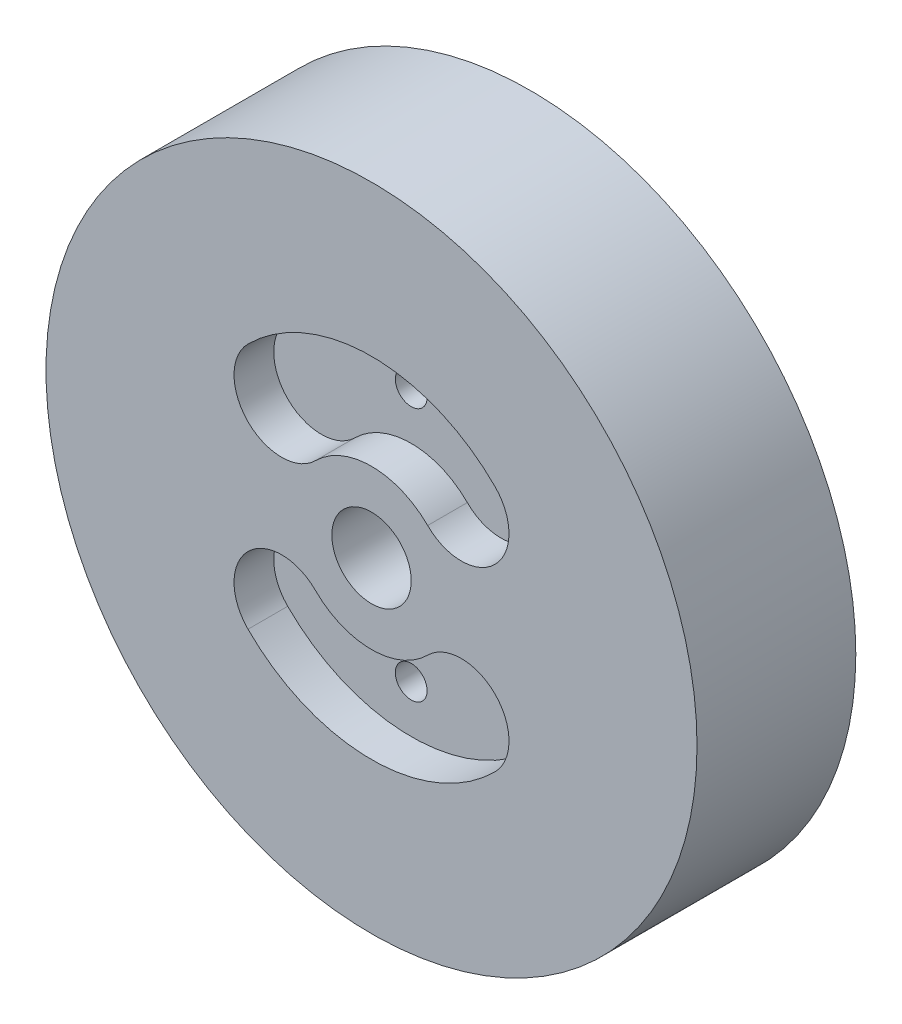
ISO-10303-21;
HEADER;
FILE_DESCRIPTION(('STEP AP214'),'2;1');
FILE_NAME('part.step','',(''),(''),'','','');
FILE_SCHEMA(('AUTOMOTIVE_DESIGN { 1 0 10303 214 1 1 1 1 }'));
ENDSEC;
DATA;
#1=APPLICATION_CONTEXT('core data for automotive mechanical design processes');
#2=APPLICATION_PROTOCOL_DEFINITION('international standard','automotive_design',2000,#1);
#3=PRODUCT_CONTEXT('',#1,'mechanical');
#4=PRODUCT('Part','Part','',(#3));
#5=PRODUCT_RELATED_PRODUCT_CATEGORY('part','',(#4));
#6=PRODUCT_DEFINITION_FORMATION('','',#4);
#7=PRODUCT_DEFINITION_CONTEXT('part definition',#1,'design');
#8=PRODUCT_DEFINITION('design','',#6,#7);
#9=PRODUCT_DEFINITION_SHAPE('','',#8);
#10=(LENGTH_UNIT() NAMED_UNIT(*) SI_UNIT(.MILLI.,.METRE.));
#11=(NAMED_UNIT(*) PLANE_ANGLE_UNIT() SI_UNIT($,.RADIAN.));
#12=(NAMED_UNIT(*) SI_UNIT($,.STERADIAN.) SOLID_ANGLE_UNIT());
#13=UNCERTAINTY_MEASURE_WITH_UNIT(LENGTH_MEASURE(1.E-05),#10,'distance_accuracy_value','');
#14=(GEOMETRIC_REPRESENTATION_CONTEXT(3) GLOBAL_UNCERTAINTY_ASSIGNED_CONTEXT((#13)) GLOBAL_UNIT_ASSIGNED_CONTEXT((#10,
#11,#12)) REPRESENTATION_CONTEXT('',''));
#15=CARTESIAN_POINT('',(0.,0.,0.));
#16=DIRECTION('',(0.,0.,1.));
#17=DIRECTION('',(1.,0.,0.));
#18=AXIS2_PLACEMENT_3D('',#15,#16,#17);
#19=CARTESIAN_POINT('',(0.,0.,10.));
#20=DIRECTION('',(0.,0.,-1.));
#21=DIRECTION('',(-1.,0.,0.));
#22=AXIS2_PLACEMENT_3D('',#19,#20,#21);
#23=CYLINDRICAL_SURFACE('',#22,20.5);
#24=CARTESIAN_POINT('',(0.,0.,10.));
#25=DIRECTION('',(0.,0.,1.));
#26=DIRECTION('',(1.,0.,0.));
#27=AXIS2_PLACEMENT_3D('',#24,#25,#26);
#28=CIRCLE('',#27,20.5);
#29=CARTESIAN_POINT('',(20.5,0.,10.));
#30=VERTEX_POINT('',#29);
#31=EDGE_CURVE('E11',#30,#30,#28,.T.);
#32=ORIENTED_EDGE('',*,*,#31,.F.);
#33=EDGE_LOOP('',(#32));
#34=FACE_BOUND('',#33,.T.);
#35=CARTESIAN_POINT('',(0.,0.,0.));
#36=DIRECTION('',(0.,0.,1.));
#37=DIRECTION('',(1.,0.,0.));
#38=AXIS2_PLACEMENT_3D('',#35,#36,#37);
#39=CIRCLE('',#38,20.5);
#40=CARTESIAN_POINT('',(20.5,0.,0.));
#41=VERTEX_POINT('',#40);
#42=EDGE_CURVE('E52',#41,#41,#39,.T.);
#43=ORIENTED_EDGE('',*,*,#42,.T.);
#44=EDGE_LOOP('',(#43));
#45=FACE_BOUND('',#44,.T.);
#46=ADVANCED_FACE('F44',(#34,#45),#23,.T.);
#47=CARTESIAN_POINT('',(0.,0.,10.));
#48=DIRECTION('',(0.,0.,1.));
#49=DIRECTION('',(1.,0.,0.));
#50=AXIS2_PLACEMENT_3D('',#47,#48,#49);
#51=PLANE('',#50);
#52=CARTESIAN_POINT('',(0.,0.,10.));
#53=DIRECTION('',(0.,0.,1.));
#54=DIRECTION('',(1.,0.,0.));
#55=AXIS2_PLACEMENT_3D('',#52,#53,#54);
#56=CIRCLE('',#55,2.5);
#57=CARTESIAN_POINT('',(2.5,0.,10.));
#58=VERTEX_POINT('',#57);
#59=EDGE_CURVE('E190',#58,#58,#56,.T.);
#60=ORIENTED_EDGE('',*,*,#59,.F.);
#61=EDGE_LOOP('',(#60));
#62=FACE_BOUND('',#61,.T.);
#63=CARTESIAN_POINT('',(5.65685424949237,-5.65685424949239,10.));
#64=DIRECTION('',(0.,0.,1.));
#65=DIRECTION('',(-1.,0.,0.));
#66=AXIS2_PLACEMENT_3D('',#63,#64,#65);
#67=CIRCLE('',#66,3.);
#68=CARTESIAN_POINT('',(7.77817459305201,-7.77817459305204,10.));
#69=VERTEX_POINT('',#68);
#70=CARTESIAN_POINT('',(3.53553390593273,-3.53553390593274,10.));
#71=VERTEX_POINT('',#70);
#72=EDGE_CURVE('E61',#69,#71,#67,.T.);
#73=ORIENTED_EDGE('',*,*,#72,.F.);
#74=CARTESIAN_POINT('',(0.,0.,10.));
#75=DIRECTION('',(0.,0.,1.));
#76=DIRECTION('',(-1.,0.,0.));
#77=AXIS2_PLACEMENT_3D('',#74,#75,#76);
#78=CIRCLE('',#77,11.);
#79=CARTESIAN_POINT('',(-7.77817459305201,-7.77817459305204,10.));
#80=VERTEX_POINT('',#79);
#81=EDGE_CURVE('E131',#80,#69,#78,.T.);
#82=ORIENTED_EDGE('',*,*,#81,.F.);
#83=CARTESIAN_POINT('',(-5.65685424949237,-5.65685424949239,10.));
#84=DIRECTION('',(0.,0.,1.));
#85=DIRECTION('',(1.,0.,0.));
#86=AXIS2_PLACEMENT_3D('',#83,#84,#85);
#87=CIRCLE('',#86,3.);
#88=CARTESIAN_POINT('',(-3.53553390593273,-3.53553390593275,10.));
#89=VERTEX_POINT('',#88);
#90=EDGE_CURVE('E133',#89,#80,#87,.T.);
#91=ORIENTED_EDGE('',*,*,#90,.F.);
#92=CARTESIAN_POINT('',(0.,0.,10.));
#93=DIRECTION('',(0.,0.,-1.));
#94=DIRECTION('',(-1.,0.,0.));
#95=AXIS2_PLACEMENT_3D('',#92,#93,#94);
#96=CIRCLE('',#95,5.);
#97=EDGE_CURVE('E141',#71,#89,#96,.T.);
#98=ORIENTED_EDGE('',*,*,#97,.F.);
#99=EDGE_LOOP('',(#73,#82,#91,#98));
#100=FACE_BOUND('',#99,.T.);
#101=CARTESIAN_POINT('',(5.65685424949237,5.65685424949239,10.));
#102=DIRECTION('',(0.,0.,1.));
#103=DIRECTION('',(1.,0.,0.));
#104=AXIS2_PLACEMENT_3D('',#101,#102,#103);
#105=CIRCLE('',#104,3.);
#106=CARTESIAN_POINT('',(3.53553390593273,3.53553390593274,10.));
#107=VERTEX_POINT('',#106);
#108=CARTESIAN_POINT('',(7.778174593052,7.77817459305204,10.));
#109=VERTEX_POINT('',#108);
#110=EDGE_CURVE('E66',#107,#109,#105,.T.);
#111=ORIENTED_EDGE('',*,*,#110,.F.);
#112=CARTESIAN_POINT('',(0.,0.,10.));
#113=DIRECTION('',(0.,0.,-1.));
#114=DIRECTION('',(1.,0.,0.));
#115=AXIS2_PLACEMENT_3D('',#112,#113,#114);
#116=CIRCLE('',#115,5.);
#117=CARTESIAN_POINT('',(-3.53553390593273,3.53553390593275,10.));
#118=VERTEX_POINT('',#117);
#119=EDGE_CURVE('E160',#118,#107,#116,.T.);
#120=ORIENTED_EDGE('',*,*,#119,.F.);
#121=CARTESIAN_POINT('',(-5.65685424949237,5.65685424949239,10.));
#122=DIRECTION('',(0.,0.,1.));
#123=DIRECTION('',(-1.,0.,0.));
#124=AXIS2_PLACEMENT_3D('',#121,#122,#123);
#125=CIRCLE('',#124,3.);
#126=CARTESIAN_POINT('',(-7.778174593052,7.77817459305204,10.));
#127=VERTEX_POINT('',#126);
#128=EDGE_CURVE('E171',#127,#118,#125,.T.);
#129=ORIENTED_EDGE('',*,*,#128,.F.);
#130=CARTESIAN_POINT('',(0.,0.,10.));
#131=DIRECTION('',(0.,0.,1.));
#132=DIRECTION('',(1.,0.,0.));
#133=AXIS2_PLACEMENT_3D('',#130,#131,#132);
#134=CIRCLE('',#133,11.);
#135=EDGE_CURVE('E169',#109,#127,#134,.T.);
#136=ORIENTED_EDGE('',*,*,#135,.F.);
#137=EDGE_LOOP('',(#111,#120,#129,#136));
#138=FACE_BOUND('',#137,.T.);
#139=ORIENTED_EDGE('',*,*,#31,.T.);
#140=EDGE_LOOP('',(#139));
#141=FACE_BOUND('',#140,.T.);
#142=ADVANCED_FACE('F223',(#62,#100,#138,#141),#51,.T.);
#143=CARTESIAN_POINT('',(0.,0.,0.));
#144=DIRECTION('',(0.,0.,1.));
#145=DIRECTION('',(1.,0.,0.));
#146=AXIS2_PLACEMENT_3D('',#143,#144,#145);
#147=PLANE('',#146);
#148=CARTESIAN_POINT('',(-12.5,0.,0.));
#149=DIRECTION('',(0.,0.,-1.));
#150=DIRECTION('',(-1.,0.,0.));
#151=AXIS2_PLACEMENT_3D('',#148,#149,#150);
#152=CIRCLE('',#151,2.5);
#153=CARTESIAN_POINT('',(-15.,0.,0.));
#154=VERTEX_POINT('',#153);
#155=EDGE_CURVE('E206',#154,#154,#152,.T.);
#156=ORIENTED_EDGE('',*,*,#155,.F.);
#157=EDGE_LOOP('',(#156));
#158=FACE_BOUND('',#157,.T.);
#159=CARTESIAN_POINT('',(12.5,0.,0.));
#160=DIRECTION('',(0.,0.,-1.));
#161=DIRECTION('',(-1.,0.,0.));
#162=AXIS2_PLACEMENT_3D('',#159,#160,#161);
#163=CIRCLE('',#162,2.5);
#164=CARTESIAN_POINT('',(10.,0.,0.));
#165=VERTEX_POINT('',#164);
#166=EDGE_CURVE('E199',#165,#165,#163,.T.);
#167=ORIENTED_EDGE('',*,*,#166,.F.);
#168=EDGE_LOOP('',(#167));
#169=FACE_BOUND('',#168,.T.);
#170=CARTESIAN_POINT('',(0.,-8.,0.));
#171=DIRECTION('',(0.,0.,1.));
#172=DIRECTION('',(1.,0.,0.));
#173=AXIS2_PLACEMENT_3D('',#170,#171,#172);
#174=CIRCLE('',#173,1.);
#175=CARTESIAN_POINT('',(1.,-8.,0.));
#176=VERTEX_POINT('',#175);
#177=EDGE_CURVE('E186',#176,#176,#174,.T.);
#178=ORIENTED_EDGE('',*,*,#177,.T.);
#179=EDGE_LOOP('',(#178));
#180=FACE_BOUND('',#179,.T.);
#181=CARTESIAN_POINT('',(0.,8.,0.));
#182=DIRECTION('',(0.,0.,1.));
#183=DIRECTION('',(1.,0.,0.));
#184=AXIS2_PLACEMENT_3D('',#181,#182,#183);
#185=CIRCLE('',#184,1.);
#186=CARTESIAN_POINT('',(1.,8.,0.));
#187=VERTEX_POINT('',#186);
#188=EDGE_CURVE('E139',#187,#187,#185,.T.);
#189=ORIENTED_EDGE('',*,*,#188,.T.);
#190=EDGE_LOOP('',(#189));
#191=FACE_BOUND('',#190,.T.);
#192=CARTESIAN_POINT('',(0.,0.,0.));
#193=DIRECTION('',(0.,0.,1.));
#194=DIRECTION('',(1.,0.,0.));
#195=AXIS2_PLACEMENT_3D('',#192,#193,#194);
#196=CIRCLE('',#195,2.5);
#197=CARTESIAN_POINT('',(2.5,0.,0.));
#198=VERTEX_POINT('',#197);
#199=EDGE_CURVE('E48',#198,#198,#196,.T.);
#200=ORIENTED_EDGE('',*,*,#199,.T.);
#201=EDGE_LOOP('',(#200));
#202=FACE_BOUND('',#201,.T.);
#203=ORIENTED_EDGE('',*,*,#42,.F.);
#204=EDGE_LOOP('',(#203));
#205=FACE_BOUND('',#204,.T.);
#206=ADVANCED_FACE('F222',(#158,#169,#180,#191,#202,#205),#147,.F.);
#207=CARTESIAN_POINT('',(5.65685424949237,5.65685424949239,7.5));
#208=DIRECTION('',(0.,0.,1.));
#209=DIRECTION('',(1.,0.,0.));
#210=AXIS2_PLACEMENT_3D('',#207,#208,#209);
#211=CYLINDRICAL_SURFACE('',#210,3.);
#212=ORIENTED_EDGE('',*,*,#110,.T.);
#213=DIRECTION('',(0.,0.,1.));
#214=VECTOR('',#213,1.);
#215=CARTESIAN_POINT('',(7.778174593052,7.77817459305204,7.5));
#216=LINE('',#215,#214);
#217=CARTESIAN_POINT('',(7.778174593052,7.77817459305204,7.5));
#218=VERTEX_POINT('',#217);
#219=EDGE_CURVE('E167',#218,#109,#216,.T.);
#220=ORIENTED_EDGE('',*,*,#219,.F.);
#221=CARTESIAN_POINT('',(5.65685424949237,5.65685424949239,7.5));
#222=DIRECTION('',(0.,0.,1.));
#223=DIRECTION('',(1.,0.,0.));
#224=AXIS2_PLACEMENT_3D('',#221,#222,#223);
#225=CIRCLE('',#224,3.);
#226=CARTESIAN_POINT('',(3.53553390593273,3.53553390593274,7.5));
#227=VERTEX_POINT('',#226);
#228=EDGE_CURVE('E153',#227,#218,#225,.T.);
#229=ORIENTED_EDGE('',*,*,#228,.F.);
#230=DIRECTION('',(0.,0.,1.));
#231=VECTOR('',#230,1.);
#232=CARTESIAN_POINT('',(3.53553390593273,3.53553390593274,7.5));
#233=LINE('',#232,#231);
#234=EDGE_CURVE('E145',#227,#107,#233,.T.);
#235=ORIENTED_EDGE('',*,*,#234,.T.);
#236=EDGE_LOOP('',(#212,#220,#229,#235));
#237=FACE_BOUND('',#236,.T.);
#238=ADVANCED_FACE('F221',(#237),#211,.F.);
#239=CARTESIAN_POINT('',(0.,0.,7.5));
#240=DIRECTION('',(0.,0.,1.));
#241=DIRECTION('',(1.,0.,0.));
#242=AXIS2_PLACEMENT_3D('',#239,#240,#241);
#243=CYLINDRICAL_SURFACE('',#242,5.);
#244=ORIENTED_EDGE('',*,*,#119,.T.);
#245=ORIENTED_EDGE('',*,*,#234,.F.);
#246=CARTESIAN_POINT('',(0.,0.,7.5));
#247=DIRECTION('',(0.,0.,-1.));
#248=DIRECTION('',(1.,0.,0.));
#249=AXIS2_PLACEMENT_3D('',#246,#247,#248);
#250=CIRCLE('',#249,5.);
#251=CARTESIAN_POINT('',(-3.53553390593273,3.53553390593275,7.5));
#252=VERTEX_POINT('',#251);
#253=EDGE_CURVE('E162',#252,#227,#250,.T.);
#254=ORIENTED_EDGE('',*,*,#253,.F.);
#255=DIRECTION('',(0.,0.,1.));
#256=VECTOR('',#255,1.);
#257=CARTESIAN_POINT('',(-3.53553390593273,3.53553390593275,7.5));
#258=LINE('',#257,#256);
#259=EDGE_CURVE('E179',#252,#118,#258,.T.);
#260=ORIENTED_EDGE('',*,*,#259,.T.);
#261=EDGE_LOOP('',(#244,#245,#254,#260));
#262=FACE_BOUND('',#261,.T.);
#263=ADVANCED_FACE('F255',(#262),#243,.T.);
#264=CARTESIAN_POINT('',(-5.65685424949237,5.65685424949239,7.5));
#265=DIRECTION('',(0.,0.,1.));
#266=DIRECTION('',(1.,0.,0.));
#267=AXIS2_PLACEMENT_3D('',#264,#265,#266);
#268=CYLINDRICAL_SURFACE('',#267,3.);
#269=ORIENTED_EDGE('',*,*,#128,.T.);
#270=ORIENTED_EDGE('',*,*,#259,.F.);
#271=CARTESIAN_POINT('',(-5.65685424949237,5.65685424949239,7.5));
#272=DIRECTION('',(0.,0.,1.));
#273=DIRECTION('',(-1.,0.,0.));
#274=AXIS2_PLACEMENT_3D('',#271,#272,#273);
#275=CIRCLE('',#274,3.);
#276=CARTESIAN_POINT('',(-7.778174593052,7.77817459305204,7.5));
#277=VERTEX_POINT('',#276);
#278=EDGE_CURVE('E159',#277,#252,#275,.T.);
#279=ORIENTED_EDGE('',*,*,#278,.F.);
#280=DIRECTION('',(0.,0.,1.));
#281=VECTOR('',#280,1.);
#282=CARTESIAN_POINT('',(-7.778174593052,7.77817459305204,7.5));
#283=LINE('',#282,#281);
#284=EDGE_CURVE('E176',#277,#127,#283,.T.);
#285=ORIENTED_EDGE('',*,*,#284,.T.);
#286=EDGE_LOOP('',(#269,#270,#279,#285));
#287=FACE_BOUND('',#286,.T.);
#288=ADVANCED_FACE('F259',(#287),#268,.F.);
#289=CARTESIAN_POINT('',(0.,0.,7.5));
#290=DIRECTION('',(0.,0.,1.));
#291=DIRECTION('',(1.,0.,0.));
#292=AXIS2_PLACEMENT_3D('',#289,#290,#291);
#293=CYLINDRICAL_SURFACE('',#292,11.);
#294=ORIENTED_EDGE('',*,*,#135,.T.);
#295=ORIENTED_EDGE('',*,*,#284,.F.);
#296=CARTESIAN_POINT('',(0.,0.,7.5));
#297=DIRECTION('',(0.,0.,1.));
#298=DIRECTION('',(1.,0.,0.));
#299=AXIS2_PLACEMENT_3D('',#296,#297,#298);
#300=CIRCLE('',#299,11.);
#301=EDGE_CURVE('E156',#218,#277,#300,.T.);
#302=ORIENTED_EDGE('',*,*,#301,.F.);
#303=ORIENTED_EDGE('',*,*,#219,.T.);
#304=EDGE_LOOP('',(#294,#295,#302,#303));
#305=FACE_BOUND('',#304,.T.);
#306=ADVANCED_FACE('F254',(#305),#293,.F.);
#307=CARTESIAN_POINT('',(2.82842712474618,2.8284271247462,7.5));
#308=DIRECTION('',(0.,0.,1.));
#309=DIRECTION('',(1.,0.,0.));
#310=AXIS2_PLACEMENT_3D('',#307,#308,#309);
#311=PLANE('',#310);
#312=CARTESIAN_POINT('',(0.,8.,7.5));
#313=DIRECTION('',(0.,0.,1.));
#314=DIRECTION('',(1.,0.,0.));
#315=AXIS2_PLACEMENT_3D('',#312,#313,#314);
#316=CIRCLE('',#315,1.);
#317=CARTESIAN_POINT('',(1.,8.,7.5));
#318=VERTEX_POINT('',#317);
#319=EDGE_CURVE('E187',#318,#318,#316,.T.);
#320=ORIENTED_EDGE('',*,*,#319,.F.);
#321=EDGE_LOOP('',(#320));
#322=FACE_BOUND('',#321,.T.);
#323=ORIENTED_EDGE('',*,*,#228,.T.);
#324=ORIENTED_EDGE('',*,*,#301,.T.);
#325=ORIENTED_EDGE('',*,*,#278,.T.);
#326=ORIENTED_EDGE('',*,*,#253,.T.);
#327=EDGE_LOOP('',(#323,#324,#325,#326));
#328=FACE_BOUND('',#327,.T.);
#329=ADVANCED_FACE('F256',(#322,#328),#311,.T.);
#330=CARTESIAN_POINT('',(5.65685424949237,-5.65685424949239,7.5));
#331=DIRECTION('',(0.,0.,1.));
#332=DIRECTION('',(1.,0.,0.));
#333=AXIS2_PLACEMENT_3D('',#330,#331,#332);
#334=CYLINDRICAL_SURFACE('',#333,3.);
#335=ORIENTED_EDGE('',*,*,#72,.T.);
#336=DIRECTION('',(0.,0.,1.));
#337=VECTOR('',#336,1.);
#338=CARTESIAN_POINT('',(3.53553390593273,-3.53553390593274,7.5));
#339=LINE('',#338,#337);
#340=CARTESIAN_POINT('',(3.53553390593273,-3.53553390593274,7.5));
#341=VERTEX_POINT('',#340);
#342=EDGE_CURVE('E108',#341,#71,#339,.T.);
#343=ORIENTED_EDGE('',*,*,#342,.F.);
#344=CARTESIAN_POINT('',(5.65685424949237,-5.65685424949239,7.5));
#345=DIRECTION('',(0.,0.,1.));
#346=DIRECTION('',(-1.,0.,0.));
#347=AXIS2_PLACEMENT_3D('',#344,#345,#346);
#348=CIRCLE('',#347,3.);
#349=CARTESIAN_POINT('',(7.77817459305201,-7.77817459305204,7.5));
#350=VERTEX_POINT('',#349);
#351=EDGE_CURVE('E114',#350,#341,#348,.T.);
#352=ORIENTED_EDGE('',*,*,#351,.F.);
#353=DIRECTION('',(0.,0.,1.));
#354=VECTOR('',#353,1.);
#355=CARTESIAN_POINT('',(7.77817459305201,-7.77817459305204,7.5));
#356=LINE('',#355,#354);
#357=EDGE_CURVE('E146',#350,#69,#356,.T.);
#358=ORIENTED_EDGE('',*,*,#357,.T.);
#359=EDGE_LOOP('',(#335,#343,#352,#358));
#360=FACE_BOUND('',#359,.T.);
#361=ADVANCED_FACE('F112',(#360),#334,.F.);
#362=CARTESIAN_POINT('',(0.,0.,7.5));
#363=DIRECTION('',(0.,0.,1.));
#364=DIRECTION('',(1.,0.,0.));
#365=AXIS2_PLACEMENT_3D('',#362,#363,#364);
#366=CYLINDRICAL_SURFACE('',#365,11.);
#367=ORIENTED_EDGE('',*,*,#81,.T.);
#368=ORIENTED_EDGE('',*,*,#357,.F.);
#369=CARTESIAN_POINT('',(0.,0.,7.5));
#370=DIRECTION('',(0.,0.,1.));
#371=DIRECTION('',(-1.,0.,0.));
#372=AXIS2_PLACEMENT_3D('',#369,#370,#371);
#373=CIRCLE('',#372,11.);
#374=CARTESIAN_POINT('',(-7.77817459305201,-7.77817459305204,7.5));
#375=VERTEX_POINT('',#374);
#376=EDGE_CURVE('E118',#375,#350,#373,.T.);
#377=ORIENTED_EDGE('',*,*,#376,.F.);
#378=DIRECTION('',(0.,0.,1.));
#379=VECTOR('',#378,1.);
#380=CARTESIAN_POINT('',(-7.77817459305201,-7.77817459305204,7.5));
#381=LINE('',#380,#379);
#382=EDGE_CURVE('E147',#375,#80,#381,.T.);
#383=ORIENTED_EDGE('',*,*,#382,.T.);
#384=EDGE_LOOP('',(#367,#368,#377,#383));
#385=FACE_BOUND('',#384,.T.);
#386=ADVANCED_FACE('F275',(#385),#366,.F.);
#387=CARTESIAN_POINT('',(-5.65685424949237,-5.65685424949239,7.5));
#388=DIRECTION('',(0.,0.,1.));
#389=DIRECTION('',(1.,0.,0.));
#390=AXIS2_PLACEMENT_3D('',#387,#388,#389);
#391=CYLINDRICAL_SURFACE('',#390,3.);
#392=ORIENTED_EDGE('',*,*,#90,.T.);
#393=ORIENTED_EDGE('',*,*,#382,.F.);
#394=CARTESIAN_POINT('',(-5.65685424949237,-5.65685424949239,7.5));
#395=DIRECTION('',(0.,0.,1.));
#396=DIRECTION('',(1.,0.,0.));
#397=AXIS2_PLACEMENT_3D('',#394,#395,#396);
#398=CIRCLE('',#397,3.);
#399=CARTESIAN_POINT('',(-3.53553390593273,-3.53553390593275,7.5));
#400=VERTEX_POINT('',#399);
#401=EDGE_CURVE('E130',#400,#375,#398,.T.);
#402=ORIENTED_EDGE('',*,*,#401,.F.);
#403=DIRECTION('',(0.,0.,1.));
#404=VECTOR('',#403,1.);
#405=CARTESIAN_POINT('',(-3.53553390593273,-3.53553390593275,7.5));
#406=LINE('',#405,#404);
#407=EDGE_CURVE('E117',#400,#89,#406,.T.);
#408=ORIENTED_EDGE('',*,*,#407,.T.);
#409=EDGE_LOOP('',(#392,#393,#402,#408));
#410=FACE_BOUND('',#409,.T.);
#411=ADVANCED_FACE('F273',(#410),#391,.F.);
#412=CARTESIAN_POINT('',(0.,0.,7.5));
#413=DIRECTION('',(0.,0.,1.));
#414=DIRECTION('',(1.,0.,0.));
#415=AXIS2_PLACEMENT_3D('',#412,#413,#414);
#416=CYLINDRICAL_SURFACE('',#415,5.);
#417=ORIENTED_EDGE('',*,*,#97,.T.);
#418=ORIENTED_EDGE('',*,*,#407,.F.);
#419=CARTESIAN_POINT('',(0.,0.,7.5));
#420=DIRECTION('',(0.,0.,-1.));
#421=DIRECTION('',(-1.,0.,0.));
#422=AXIS2_PLACEMENT_3D('',#419,#420,#421);
#423=CIRCLE('',#422,5.);
#424=EDGE_CURVE('E124',#341,#400,#423,.T.);
#425=ORIENTED_EDGE('',*,*,#424,.F.);
#426=ORIENTED_EDGE('',*,*,#342,.T.);
#427=EDGE_LOOP('',(#417,#418,#425,#426));
#428=FACE_BOUND('',#427,.T.);
#429=ADVANCED_FACE('F125',(#428),#416,.T.);
#430=CARTESIAN_POINT('',(2.82842712474618,-2.8284271247462,7.5));
#431=DIRECTION('',(0.,0.,-1.));
#432=DIRECTION('',(-1.,0.,0.));
#433=AXIS2_PLACEMENT_3D('',#430,#431,#432);
#434=PLANE('',#433);
#435=CARTESIAN_POINT('',(0.,-8.,7.5));
#436=DIRECTION('',(0.,0.,-1.));
#437=DIRECTION('',(-1.,0.,0.));
#438=AXIS2_PLACEMENT_3D('',#435,#436,#437);
#439=CIRCLE('',#438,1.);
#440=CARTESIAN_POINT('',(-1.,-8.,7.5));
#441=VERTEX_POINT('',#440);
#442=EDGE_CURVE('E184',#441,#441,#439,.T.);
#443=ORIENTED_EDGE('',*,*,#442,.T.);
#444=EDGE_LOOP('',(#443));
#445=FACE_BOUND('',#444,.T.);
#446=ORIENTED_EDGE('',*,*,#351,.T.);
#447=ORIENTED_EDGE('',*,*,#424,.T.);
#448=ORIENTED_EDGE('',*,*,#401,.T.);
#449=ORIENTED_EDGE('',*,*,#376,.T.);
#450=EDGE_LOOP('',(#446,#447,#448,#449));
#451=FACE_BOUND('',#450,.T.);
#452=ADVANCED_FACE('F129',(#445,#451),#434,.F.);
#453=CARTESIAN_POINT('',(0.,-8.,-22.5));
#454=DIRECTION('',(0.,0.,1.));
#455=DIRECTION('',(1.,0.,0.));
#456=AXIS2_PLACEMENT_3D('',#453,#454,#455);
#457=CYLINDRICAL_SURFACE('',#456,1.);
#458=ORIENTED_EDGE('',*,*,#442,.F.);
#459=EDGE_LOOP('',(#458));
#460=FACE_BOUND('',#459,.T.);
#461=ORIENTED_EDGE('',*,*,#177,.F.);
#462=EDGE_LOOP('',(#461));
#463=FACE_BOUND('',#462,.T.);
#464=ADVANCED_FACE('F282',(#460,#463),#457,.F.);
#465=CARTESIAN_POINT('',(0.,8.,-22.5));
#466=DIRECTION('',(0.,0.,1.));
#467=DIRECTION('',(1.,0.,0.));
#468=AXIS2_PLACEMENT_3D('',#465,#466,#467);
#469=CYLINDRICAL_SURFACE('',#468,1.);
#470=ORIENTED_EDGE('',*,*,#319,.T.);
#471=EDGE_LOOP('',(#470));
#472=FACE_BOUND('',#471,.T.);
#473=ORIENTED_EDGE('',*,*,#188,.F.);
#474=EDGE_LOOP('',(#473));
#475=FACE_BOUND('',#474,.T.);
#476=ADVANCED_FACE('F286',(#472,#475),#469,.F.);
#477=CARTESIAN_POINT('',(0.,0.,-22.5));
#478=DIRECTION('',(0.,0.,1.));
#479=DIRECTION('',(1.,0.,0.));
#480=AXIS2_PLACEMENT_3D('',#477,#478,#479);
#481=CYLINDRICAL_SURFACE('',#480,2.5);
#482=ORIENTED_EDGE('',*,*,#59,.T.);
#483=EDGE_LOOP('',(#482));
#484=FACE_BOUND('',#483,.T.);
#485=ORIENTED_EDGE('',*,*,#199,.F.);
#486=EDGE_LOOP('',(#485));
#487=FACE_BOUND('',#486,.T.);
#488=ADVANCED_FACE('F284',(#484,#487),#481,.F.);
#489=CARTESIAN_POINT('',(12.5,0.,5.));
#490=DIRECTION('',(0.,0.,-1.));
#491=DIRECTION('',(-1.,0.,0.));
#492=AXIS2_PLACEMENT_3D('',#489,#490,#491);
#493=CYLINDRICAL_SURFACE('',#492,2.5);
#494=CARTESIAN_POINT('',(12.5,0.,5.));
#495=DIRECTION('',(0.,0.,-1.));
#496=DIRECTION('',(-1.,0.,0.));
#497=AXIS2_PLACEMENT_3D('',#494,#495,#496);
#498=CIRCLE('',#497,2.5);
#499=CARTESIAN_POINT('',(10.,0.,5.));
#500=VERTEX_POINT('',#499);
#501=EDGE_CURVE('E201',#500,#500,#498,.T.);
#502=ORIENTED_EDGE('',*,*,#501,.F.);
#503=EDGE_LOOP('',(#502));
#504=FACE_BOUND('',#503,.T.);
#505=ORIENTED_EDGE('',*,*,#166,.T.);
#506=EDGE_LOOP('',(#505));
#507=FACE_BOUND('',#506,.T.);
#508=ADVANCED_FACE('F290',(#504,#507),#493,.F.);
#509=CARTESIAN_POINT('',(12.5,0.,5.));
#510=DIRECTION('',(0.,0.,-1.));
#511=DIRECTION('',(-1.,0.,0.));
#512=AXIS2_PLACEMENT_3D('',#509,#510,#511);
#513=PLANE('',#512);
#514=ORIENTED_EDGE('',*,*,#501,.T.);
#515=EDGE_LOOP('',(#514));
#516=FACE_BOUND('',#515,.T.);
#517=ADVANCED_FACE('F220',(#516),#513,.T.);
#518=CARTESIAN_POINT('',(-12.5,0.,5.));
#519=DIRECTION('',(0.,0.,-1.));
#520=DIRECTION('',(-1.,0.,0.));
#521=AXIS2_PLACEMENT_3D('',#518,#519,#520);
#522=CYLINDRICAL_SURFACE('',#521,2.5);
#523=CARTESIAN_POINT('',(-12.5,0.,5.));
#524=DIRECTION('',(0.,0.,-1.));
#525=DIRECTION('',(-1.,0.,0.));
#526=AXIS2_PLACEMENT_3D('',#523,#524,#525);
#527=CIRCLE('',#526,2.5);
#528=CARTESIAN_POINT('',(-15.,0.,5.));
#529=VERTEX_POINT('',#528);
#530=EDGE_CURVE('E200',#529,#529,#527,.T.);
#531=ORIENTED_EDGE('',*,*,#530,.F.);
#532=EDGE_LOOP('',(#531));
#533=FACE_BOUND('',#532,.T.);
#534=ORIENTED_EDGE('',*,*,#155,.T.);
#535=EDGE_LOOP('',(#534));
#536=FACE_BOUND('',#535,.T.);
#537=ADVANCED_FACE('F212',(#533,#536),#522,.F.);
#538=CARTESIAN_POINT('',(-12.5,0.,5.));
#539=DIRECTION('',(0.,0.,-1.));
#540=DIRECTION('',(-1.,0.,0.));
#541=AXIS2_PLACEMENT_3D('',#538,#539,#540);
#542=PLANE('',#541);
#543=ORIENTED_EDGE('',*,*,#530,.T.);
#544=EDGE_LOOP('',(#543));
#545=FACE_BOUND('',#544,.T.);
#546=ADVANCED_FACE('F215',(#545),#542,.T.);
#547=CLOSED_SHELL('',(#46,#142,#206,#238,#263,#288,#306,#329,#361,#386,#411,#429,#452,#464,#476,
#488,#508,#517,#537,#546));
#548=MANIFOLD_SOLID_BREP('B2',#547);
#549=ADVANCED_BREP_SHAPE_REPRESENTATION('',(#18,#548),#14);
#550=SHAPE_DEFINITION_REPRESENTATION(#9,#549);
ENDSEC;
END-ISO-10303-21;
